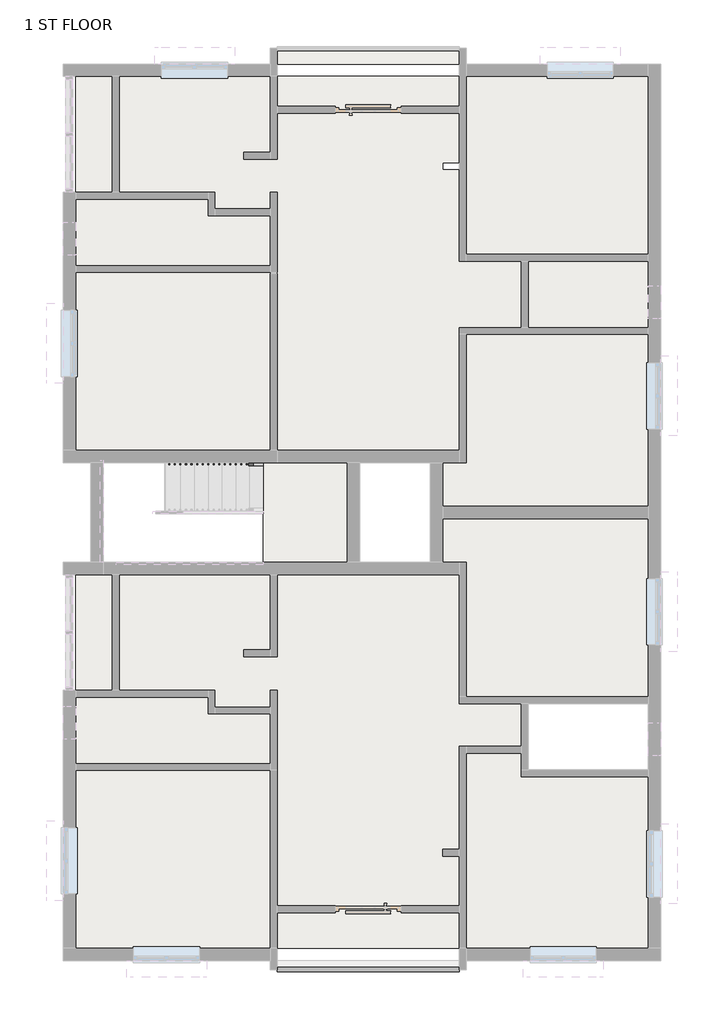
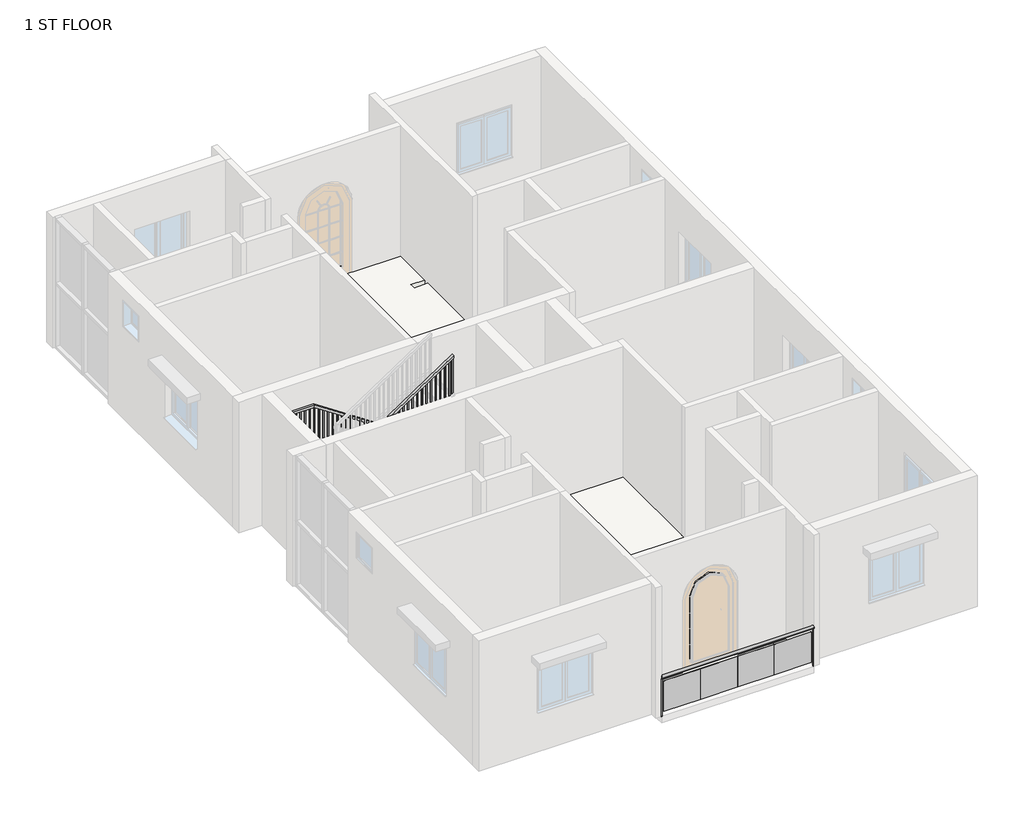
# One storey, part 3 of 4: 4 slabs, 2 railings.
"""IFC4 building model written with IfcOpenShell, lengths in millimetres."""

from ifc_helpers import new_model, si_unit, point, frame, origin, place, context, project, spatial, polyline, ellipse_curve, trimmed, outline, extrude, faceted_brep, element, save
from ifc_brep_helpers import plane_surface, extruded_surface, advanced_brep

model = new_model("IFC4")

# Units and contexts
model_context = context("Model", 3, world=origin())
ifc_project = project(units=[si_unit("LENGTHUNIT", "METRE", prefix="MILLI")], contexts=[model_context])

# Site, building, storey
site = spatial("IfcSite", under=ifc_project)
building = spatial("IfcBuilding", under=site)
storey = spatial("IfcBuildingStorey", under=building, Name="1 ST FLOOR", Elevation=6096.0)

# Railings
placement = place(None, origin())
element("IfcRailing", 1, ObjectType="Glass Panel - Bottom Fill 2", at=placement, inside=storey, context=model_context, shape_type="SolidModel", body=[
    advanced_brep(
    [(-2494.0012202, -3358.1292559, 7010.4), (-2494.0012202, -3434.3292559, 7010.4), (858.7987798, -3358.1292559, 7010.4), (858.7987798, -3434.3292559, 7010.4)],
    [
        (0, 1, ellipse_curve(frame((-2494.0012202, -3396.2292559, 7010.4), z_axis=(-1.0, 0.0, 0.0), x_axis=(0.0, -1.0, 0.0)), 38.1, 28.575)),
        (1, 0, ellipse_curve(frame((-2494.0012202, -3396.2292559, 7010.4), z_axis=(-1.0, 0.0, 0.0), x_axis=(0.0, -1.0, 0.0)), 38.1, 28.575)),
        (2, 3, ellipse_curve(frame((858.7987798, -3396.2292559, 7010.4), z_axis=(1.0, 0.0, 0.0), x_axis=(0.0, -1.0, 0.0)), 38.1, 28.575)),
        (3, 2, ellipse_curve(frame((858.7987798, -3396.2292559, 7010.4), z_axis=(1.0, 0.0, 0.0), x_axis=(0.0, -1.0, 0.0)), 38.1, 28.575)),
        (0, 2),
        (3, 1),
    ],
    [
        plane_surface(frame((-2494.0012202, -3396.2292559, 7010.4), z_axis=(-1.0, 0.0, 0.0), x_axis=(0.0, 1.0, 0.0))),
        plane_surface(frame((858.7987798, -3396.2292559, 7010.4), z_axis=(1.0, 0.0, 0.0), x_axis=(0.0, 1.0, 0.0))),
        extruded_surface(trimmed(ellipse_curve(frame((858.7987798, -3396.2292559, 7010.4), z_axis=(-1.0, 0.0, 0.0), x_axis=(0.0, -1.0, 0.0)), 38.1, 28.575), [point((858.7987798, -3358.1292559, 7010.4))], [point((858.7987798, -3434.3292559, 7010.4))], True, "CARTESIAN"), (-3352.7999999999997, 0.0, 0.0), 3352.7999999999997),
        extruded_surface(trimmed(ellipse_curve(frame((858.7987798, -3396.2292559, 7010.4), z_axis=(-1.0, 0.0, 0.0), x_axis=(0.0, -1.0, 0.0)), 38.1, 28.575), [point((858.7987798, -3434.3292559, 7010.4))], [point((858.7987798, -3358.1292559, 7010.4))], True, "CARTESIAN"), (-3352.7999999999997, 0.0, 0.0), 3352.7999999999997),
    ],
    [
        (0, [[1, 2]]),
        (1, [[3, 4]]),
        (2, [[-1, 5, -4, 6]]),
        (3, [[-2, -6, -3, -5]]),
    ],
),
    extrude(outline(polyline([(-4.8012202, -3402.7644129), (-4.8012202, -3396.4144129), (807.9987798, -3396.4144129), (807.9987798, -3402.7644129), (-4.8012202, -3402.7644129)])), frame((0.0, 0.0, 6197.6), z_axis=(0.0, 0.0, 1.0), x_axis=(1.0, 0.0, 0.0)), (0.0, 0.0, 1.0), 711.2),
    extrude(outline(polyline([(-817.6012202, -3402.7644129), (-817.6012202, -3396.4144129), (-4.8012202, -3396.4144129), (-4.8012202, -3402.7644129), (-817.6012202, -3402.7644129)])), frame((0.0, 0.0, 6197.6), z_axis=(0.0, 0.0, 1.0), x_axis=(1.0, 0.0, 0.0)), (0.0, 0.0, 1.0), 711.2),
    extrude(outline(polyline([(-1630.4012202, -3402.7644129), (-1630.4012202, -3396.4144129), (-817.6012202, -3396.4144129), (-817.6012202, -3402.7644129), (-1630.4012202, -3402.7644129)])), frame((0.0, 0.0, 6197.6), z_axis=(0.0, 0.0, 1.0), x_axis=(1.0, 0.0, 0.0)), (0.0, 0.0, 1.0), 711.2),
    extrude(outline(polyline([(-2443.2012202, -3402.7644129), (-2443.2012202, -3396.4144129), (-1630.4012202, -3396.4144129), (-1630.4012202, -3402.7644129), (-2443.2012202, -3402.7644129)])), frame((0.0, 0.0, 6197.6), z_axis=(0.0, 0.0, 1.0), x_axis=(1.0, 0.0, 0.0)), (0.0, 0.0, 1.0), 711.2),
    extrude(outline(polyline([(846.0987798, -3386.7042559), (865.1487798, -3386.7042559), (865.1487798, -3405.7542559), (846.0987798, -3405.7542559), (846.0987798, -3386.7042559)])), frame((0.0, 0.0, 6096.0), z_axis=(0.0, 0.0, 1.0), x_axis=(1.0, 0.0, 0.0)), (0.0, 0.0, 1.0), 885.825),
    extrude(outline(polyline([(-2500.3512202, -3386.7042559), (-2481.3012202, -3386.7042559), (-2481.3012202, -3405.7542559), (-2500.3512202, -3405.7542559), (-2500.3512202, -3386.7042559)])), frame((0.0, 0.0, 6096.0), z_axis=(0.0, 0.0, 1.0), x_axis=(1.0, 0.0, 0.0)), (0.0, 0.0, 1.0), 885.825),
])
element("IfcRailing", 2, ObjectType="Handrail - Rectangular", at=placement, inside=storey, context=model_context, shape_type="SolidModel", body=[
    faceted_brep([(-2748.0012202, 5879.8309003, 7179.7333333), (-2748.0012202, 5879.8309003, 7118.6793317), (-2748.0012202, 5930.6309003, 7118.6793317), (-2748.0012202, 5930.6309003, 7179.7333333), (-4780.0012202, 5879.8309003, 8534.4), (-4795.3822226, 5879.8309003, 8483.6), (-4795.3822226, 5930.6309003, 8483.6), (-4780.0012202, 5930.6309003, 8534.4), (-5643.6012202, 5879.8309003, 8534.4), (-5643.6012202, 5879.8309003, 8483.6), (-5694.4012202, 5930.6309003, 8483.6), (-5694.4012202, 5930.6309003, 8534.4), (-5643.6012202, 4152.6309003, 8534.4), (-5643.6012202, 4152.6309003, 8483.6), (-5694.4012202, 4101.8309003, 8483.6), (-5694.4012202, 4101.8309003, 8534.4), (-5034.0012202, 4152.6309003, 8534.4), (-5018.6202178, 4152.6309003, 8483.6), (-5018.6202178, 4101.8309003, 8483.6), (-5034.0012202, 4101.8309003, 8534.4), (-2748.0012202, 4152.6309003, 10058.4), (-2748.0012202, 4101.8309003, 10058.4), (-2748.0012202, 4101.8309003, 9997.3459984), (-2748.0012202, 4152.6309003, 9997.3459984)], [[[0, 1, 2, 3]], [[1, 0, 4, 5]], [[2, 1, 5, 6]], [[3, 2, 6, 7]], [[0, 3, 7, 4]], [[5, 4, 8, 9]], [[6, 5, 9, 10]], [[7, 6, 10, 11]], [[4, 7, 11, 8]], [[9, 8, 12, 13]], [[10, 9, 13, 14]], [[11, 10, 14, 15]], [[8, 11, 15, 12]], [[13, 12, 16, 17]], [[14, 13, 17, 18]], [[15, 14, 18, 19]], [[12, 15, 19, 16]], [[20, 21, 22, 23]], [[17, 16, 20, 23]], [[18, 17, 23, 22]], [[19, 18, 22, 21]], [[16, 19, 21, 20]]]),
    extrude(outline(polyline([(9952.8959984, -2814.6762202), (9940.1959984, -2833.7262202), (8974.6666667, -2833.7262202), (8974.6666667, -2814.6762202), (9952.8959984, -2814.6762202)])), frame((0.0, 4117.7059003, 0.0), z_axis=(0.0, 1.0, 0.0), x_axis=(0.0, 0.0, 1.0)), (0.0, 0.0, 1.0), 19.05),
    extrude(outline(polyline([(9885.1626651, -2916.2762202), (9872.4626651, -2935.3262202), (8974.6666667, -2935.3262202), (8974.6666667, -2916.2762202), (9885.1626651, -2916.2762202)])), frame((0.0, 4117.7059003, 0.0), z_axis=(0.0, 1.0, 0.0), x_axis=(0.0, 0.0, 1.0)), (0.0, 0.0, 1.0), 19.05),
    extrude(outline(polyline([(9817.4293317, -3017.8762202), (9804.7293317, -3036.9262202), (8805.3333333, -3036.9262202), (8805.3333333, -3017.8762202), (9817.4293317, -3017.8762202)])), frame((0.0, 4117.7059003, 0.0), z_axis=(0.0, 1.0, 0.0), x_axis=(0.0, 0.0, 1.0)), (0.0, 0.0, 1.0), 19.05),
    extrude(outline(polyline([(9749.6959984, -3119.4762202), (9736.9959984, -3138.5262202), (8805.3333333, -3138.5262202), (8805.3333333, -3119.4762202), (9749.6959984, -3119.4762202)])), frame((0.0, 4117.7059003, 0.0), z_axis=(0.0, 1.0, 0.0), x_axis=(0.0, 0.0, 1.0)), (0.0, 0.0, 1.0), 19.05),
    extrude(outline(polyline([(9681.9626651, -3221.0762202), (9669.2626651, -3240.1262202), (8805.3333333, -3240.1262202), (8805.3333333, -3221.0762202), (9681.9626651, -3221.0762202)])), frame((0.0, 4117.7059003, 0.0), z_axis=(0.0, 1.0, 0.0), x_axis=(0.0, 0.0, 1.0)), (0.0, 0.0, 1.0), 19.05),
    extrude(outline(polyline([(9614.2293317, -3322.6762202), (9601.5293317, -3341.7262202), (8636.0, -3341.7262202), (8636.0, -3322.6762202), (9614.2293317, -3322.6762202)])), frame((0.0, 4117.7059003, 0.0), z_axis=(0.0, 1.0, 0.0), x_axis=(0.0, 0.0, 1.0)), (0.0, 0.0, 1.0), 19.05),
    extrude(outline(polyline([(9546.4959984, -3424.2762202), (9533.7959984, -3443.3262202), (8636.0, -3443.3262202), (8636.0, -3424.2762202), (9546.4959984, -3424.2762202)])), frame((0.0, 4117.7059003, 0.0), z_axis=(0.0, 1.0, 0.0), x_axis=(0.0, 0.0, 1.0)), (0.0, 0.0, 1.0), 19.05),
    extrude(outline(polyline([(9478.7626651, -3525.8762202), (9466.0626651, -3544.9262202), (8466.6666667, -3544.9262202), (8466.6666667, -3525.8762202), (9478.7626651, -3525.8762202)])), frame((0.0, 4117.7059003, 0.0), z_axis=(0.0, 1.0, 0.0), x_axis=(0.0, 0.0, 1.0)), (0.0, 0.0, 1.0), 19.05),
    extrude(outline(polyline([(9411.0293317, -3627.4762202), (9398.3293317, -3646.5262202), (8466.6666667, -3646.5262202), (8466.6666667, -3627.4762202), (9411.0293317, -3627.4762202)])), frame((0.0, 4117.7059003, 0.0), z_axis=(0.0, 1.0, 0.0), x_axis=(0.0, 0.0, 1.0)), (0.0, 0.0, 1.0), 19.05),
    extrude(outline(polyline([(9343.2959984, -3729.0762202), (9330.5959984, -3748.1262202), (8466.6666667, -3748.1262202), (8466.6666667, -3729.0762202), (9343.2959984, -3729.0762202)])), frame((0.0, 4117.7059003, 0.0), z_axis=(0.0, 1.0, 0.0), x_axis=(0.0, 0.0, 1.0)), (0.0, 0.0, 1.0), 19.05),
    extrude(outline(polyline([(9275.5626651, -3830.6762202), (9262.8626651, -3849.7262202), (8297.3333333, -3849.7262202), (8297.3333333, -3830.6762202), (9275.5626651, -3830.6762202)])), frame((0.0, 4117.7059003, 0.0), z_axis=(0.0, 1.0, 0.0), x_axis=(0.0, 0.0, 1.0)), (0.0, 0.0, 1.0), 19.05),
    extrude(outline(polyline([(9207.8293317, -3932.2762202), (9195.1293317, -3951.3262202), (8297.3333333, -3951.3262202), (8297.3333333, -3932.2762202), (9207.8293317, -3932.2762202)])), frame((0.0, 4117.7059003, 0.0), z_axis=(0.0, 1.0, 0.0), x_axis=(0.0, 0.0, 1.0)), (0.0, 0.0, 1.0), 19.05),
    extrude(outline(polyline([(9140.0959984, -4033.8762202), (9127.3959984, -4052.9262202), (8128.0, -4052.9262202), (8128.0, -4033.8762202), (9140.0959984, -4033.8762202)])), frame((0.0, 4117.7059003, 0.0), z_axis=(0.0, 1.0, 0.0), x_axis=(0.0, 0.0, 1.0)), (0.0, 0.0, 1.0), 19.05),
    extrude(outline(polyline([(9072.3626651, -4135.4762202), (9059.6626651, -4154.5262202), (8128.0, -4154.5262202), (8128.0, -4135.4762202), (9072.3626651, -4135.4762202)])), frame((0.0, 4117.7059003, 0.0), z_axis=(0.0, 1.0, 0.0), x_axis=(0.0, 0.0, 1.0)), (0.0, 0.0, 1.0), 19.05),
    extrude(outline(polyline([(9004.6293317, -4237.0762202), (8991.9293317, -4256.1262202), (8128.0, -4256.1262202), (8128.0, -4237.0762202), (9004.6293317, -4237.0762202)])), frame((0.0, 4117.7059003, 0.0), z_axis=(0.0, 1.0, 0.0), x_axis=(0.0, 0.0, 1.0)), (0.0, 0.0, 1.0), 19.05),
    extrude(outline(polyline([(8936.8959984, -4338.6762202), (8924.1959984, -4357.7262202), (7958.6666667, -4357.7262202), (7958.6666667, -4338.6762202), (8936.8959984, -4338.6762202)])), frame((0.0, 4117.7059003, 0.0), z_axis=(0.0, 1.0, 0.0), x_axis=(0.0, 0.0, 1.0)), (0.0, 0.0, 1.0), 19.05),
    extrude(outline(polyline([(8869.1626651, -4440.2762202), (8856.4626651, -4459.3262202), (7958.6666667, -4459.3262202), (7958.6666667, -4440.2762202), (8869.1626651, -4440.2762202)])), frame((0.0, 4117.7059003, 0.0), z_axis=(0.0, 1.0, 0.0), x_axis=(0.0, 0.0, 1.0)), (0.0, 0.0, 1.0), 19.05),
    extrude(outline(polyline([(8801.4293317, -4541.8762202), (8788.7293317, -4560.9262202), (7789.3333333, -4560.9262202), (7789.3333333, -4541.8762202), (8801.4293317, -4541.8762202)])), frame((0.0, 4117.7059003, 0.0), z_axis=(0.0, 1.0, 0.0), x_axis=(0.0, 0.0, 1.0)), (0.0, 0.0, 1.0), 19.05),
    extrude(outline(polyline([(8733.6959984, -4643.4762202), (8720.9959984, -4662.5262202), (7789.3333333, -4662.5262202), (7789.3333333, -4643.4762202), (8733.6959984, -4643.4762202)])), frame((0.0, 4117.7059003, 0.0), z_axis=(0.0, 1.0, 0.0), x_axis=(0.0, 0.0, 1.0)), (0.0, 0.0, 1.0), 19.05),
    extrude(outline(polyline([(8665.9626651, -4745.0762202), (8653.2626651, -4764.1262202), (7789.3333333, -4764.1262202), (7789.3333333, -4745.0762202), (8665.9626651, -4745.0762202)])), frame((0.0, 4117.7059003, 0.0), z_axis=(0.0, 1.0, 0.0), x_axis=(0.0, 0.0, 1.0)), (0.0, 0.0, 1.0), 19.05),
    extrude(outline(polyline([(8598.2293317, -4846.6762202), (8585.5293317, -4865.7262202), (7620.0, -4865.7262202), (7620.0, -4846.6762202), (8598.2293317, -4846.6762202)])), frame((0.0, 4117.7059003, 0.0), z_axis=(0.0, 1.0, 0.0), x_axis=(0.0, 0.0, 1.0)), (0.0, 0.0, 1.0), 19.05),
    extrude(outline(polyline([(8530.4959984, -4948.2762202), (8517.7959984, -4967.3262202), (7620.0, -4967.3262202), (7620.0, -4948.2762202), (8530.4959984, -4948.2762202)])), frame((0.0, 4117.7059003, 0.0), z_axis=(0.0, 1.0, 0.0), x_axis=(0.0, 0.0, 1.0)), (0.0, 0.0, 1.0), 19.05),
    extrude(outline(polyline([(-5068.9262202, 4117.7059003), (-5068.9262202, 4136.7559003), (-5049.8762202, 4136.7559003), (-5049.8762202, 4117.7059003), (-5068.9262202, 4117.7059003)])), frame((0.0, 0.0, 7620.0), z_axis=(0.0, 0.0, 1.0), x_axis=(1.0, 0.0, 0.0)), (0.0, 0.0, 1.0), 863.6),
    extrude(outline(polyline([(-5170.5262202, 4117.7059003), (-5170.5262202, 4136.7559003), (-5151.4762202, 4136.7559003), (-5151.4762202, 4117.7059003), (-5170.5262202, 4117.7059003)])), frame((0.0, 0.0, 7620.0), z_axis=(0.0, 0.0, 1.0), x_axis=(1.0, 0.0, 0.0)), (0.0, 0.0, 1.0), 863.6),
    extrude(outline(polyline([(-5272.1262202, 4117.7059003), (-5272.1262202, 4136.7559003), (-5253.0762202, 4136.7559003), (-5253.0762202, 4117.7059003), (-5272.1262202, 4117.7059003)])), frame((0.0, 0.0, 7620.0), z_axis=(0.0, 0.0, 1.0), x_axis=(1.0, 0.0, 0.0)), (0.0, 0.0, 1.0), 863.6),
    extrude(outline(polyline([(-5373.7262202, 4117.7059003), (-5373.7262202, 4136.7559003), (-5354.6762202, 4136.7559003), (-5354.6762202, 4117.7059003), (-5373.7262202, 4117.7059003)])), frame((0.0, 0.0, 7620.0), z_axis=(0.0, 0.0, 1.0), x_axis=(1.0, 0.0, 0.0)), (0.0, 0.0, 1.0), 863.6),
    extrude(outline(polyline([(-5475.3262202, 4117.7059003), (-5475.3262202, 4136.7559003), (-5456.2762202, 4136.7559003), (-5456.2762202, 4117.7059003), (-5475.3262202, 4117.7059003)])), frame((0.0, 0.0, 7620.0), z_axis=(0.0, 0.0, 1.0), x_axis=(1.0, 0.0, 0.0)), (0.0, 0.0, 1.0), 863.6),
    extrude(outline(polyline([(-5576.9262202, 4117.7059003), (-5576.9262202, 4136.7559003), (-5557.8762202, 4136.7559003), (-5557.8762202, 4117.7059003), (-5576.9262202, 4117.7059003)])), frame((0.0, 0.0, 7620.0), z_axis=(0.0, 0.0, 1.0), x_axis=(1.0, 0.0, 0.0)), (0.0, 0.0, 1.0), 863.6),
    extrude(outline(polyline([(-5678.5262202, 4187.5559003), (-5659.4762202, 4187.5559003), (-5659.4762202, 4168.5059003), (-5678.5262202, 4168.5059003), (-5678.5262202, 4187.5559003)])), frame((0.0, 0.0, 7620.0), z_axis=(0.0, 0.0, 1.0), x_axis=(1.0, 0.0, 0.0)), (0.0, 0.0, 1.0), 863.6),
    extrude(outline(polyline([(-5678.5262202, 4289.1559003), (-5659.4762202, 4289.1559003), (-5659.4762202, 4270.1059003), (-5678.5262202, 4270.1059003), (-5678.5262202, 4289.1559003)])), frame((0.0, 0.0, 7620.0), z_axis=(0.0, 0.0, 1.0), x_axis=(1.0, 0.0, 0.0)), (0.0, 0.0, 1.0), 863.6),
    extrude(outline(polyline([(-5678.5262202, 4390.7559003), (-5659.4762202, 4390.7559003), (-5659.4762202, 4371.7059003), (-5678.5262202, 4371.7059003), (-5678.5262202, 4390.7559003)])), frame((0.0, 0.0, 7620.0), z_axis=(0.0, 0.0, 1.0), x_axis=(1.0, 0.0, 0.0)), (0.0, 0.0, 1.0), 863.6),
    extrude(outline(polyline([(-5678.5262202, 4492.3559003), (-5659.4762202, 4492.3559003), (-5659.4762202, 4473.3059003), (-5678.5262202, 4473.3059003), (-5678.5262202, 4492.3559003)])), frame((0.0, 0.0, 7620.0), z_axis=(0.0, 0.0, 1.0), x_axis=(1.0, 0.0, 0.0)), (0.0, 0.0, 1.0), 863.6),
    extrude(outline(polyline([(-5678.5262202, 4593.9559003), (-5659.4762202, 4593.9559003), (-5659.4762202, 4574.9059003), (-5678.5262202, 4574.9059003), (-5678.5262202, 4593.9559003)])), frame((0.0, 0.0, 7620.0), z_axis=(0.0, 0.0, 1.0), x_axis=(1.0, 0.0, 0.0)), (0.0, 0.0, 1.0), 863.6),
    extrude(outline(polyline([(-5678.5262202, 4695.5559003), (-5659.4762202, 4695.5559003), (-5659.4762202, 4676.5059003), (-5678.5262202, 4676.5059003), (-5678.5262202, 4695.5559003)])), frame((0.0, 0.0, 7620.0), z_axis=(0.0, 0.0, 1.0), x_axis=(1.0, 0.0, 0.0)), (0.0, 0.0, 1.0), 863.6),
    extrude(outline(polyline([(-5678.5262202, 4797.1559003), (-5659.4762202, 4797.1559003), (-5659.4762202, 4778.1059003), (-5678.5262202, 4778.1059003), (-5678.5262202, 4797.1559003)])), frame((0.0, 0.0, 7620.0), z_axis=(0.0, 0.0, 1.0), x_axis=(1.0, 0.0, 0.0)), (0.0, 0.0, 1.0), 863.6),
    extrude(outline(polyline([(-5678.5262202, 4898.7559003), (-5659.4762202, 4898.7559003), (-5659.4762202, 4879.7059003), (-5678.5262202, 4879.7059003), (-5678.5262202, 4898.7559003)])), frame((0.0, 0.0, 7620.0), z_axis=(0.0, 0.0, 1.0), x_axis=(1.0, 0.0, 0.0)), (0.0, 0.0, 1.0), 863.6),
    extrude(outline(polyline([(-5678.5262202, 5000.3559003), (-5659.4762202, 5000.3559003), (-5659.4762202, 4981.3059003), (-5678.5262202, 4981.3059003), (-5678.5262202, 5000.3559003)])), frame((0.0, 0.0, 7620.0), z_axis=(0.0, 0.0, 1.0), x_axis=(1.0, 0.0, 0.0)), (0.0, 0.0, 1.0), 863.6),
    extrude(outline(polyline([(-5678.5262202, 5101.9559003), (-5659.4762202, 5101.9559003), (-5659.4762202, 5082.9059003), (-5678.5262202, 5082.9059003), (-5678.5262202, 5101.9559003)])), frame((0.0, 0.0, 7620.0), z_axis=(0.0, 0.0, 1.0), x_axis=(1.0, 0.0, 0.0)), (0.0, 0.0, 1.0), 863.6),
    extrude(outline(polyline([(-5678.5262202, 5203.5559003), (-5659.4762202, 5203.5559003), (-5659.4762202, 5184.5059003), (-5678.5262202, 5184.5059003), (-5678.5262202, 5203.5559003)])), frame((0.0, 0.0, 7620.0), z_axis=(0.0, 0.0, 1.0), x_axis=(1.0, 0.0, 0.0)), (0.0, 0.0, 1.0), 863.6),
    extrude(outline(polyline([(-5678.5262202, 5305.1559003), (-5659.4762202, 5305.1559003), (-5659.4762202, 5286.1059003), (-5678.5262202, 5286.1059003), (-5678.5262202, 5305.1559003)])), frame((0.0, 0.0, 7620.0), z_axis=(0.0, 0.0, 1.0), x_axis=(1.0, 0.0, 0.0)), (0.0, 0.0, 1.0), 863.6),
    extrude(outline(polyline([(-5678.5262202, 5406.7559003), (-5659.4762202, 5406.7559003), (-5659.4762202, 5387.7059003), (-5678.5262202, 5387.7059003), (-5678.5262202, 5406.7559003)])), frame((0.0, 0.0, 7620.0), z_axis=(0.0, 0.0, 1.0), x_axis=(1.0, 0.0, 0.0)), (0.0, 0.0, 1.0), 863.6),
    extrude(outline(polyline([(-5678.5262202, 5508.3559003), (-5659.4762202, 5508.3559003), (-5659.4762202, 5489.3059003), (-5678.5262202, 5489.3059003), (-5678.5262202, 5508.3559003)])), frame((0.0, 0.0, 7620.0), z_axis=(0.0, 0.0, 1.0), x_axis=(1.0, 0.0, 0.0)), (0.0, 0.0, 1.0), 863.6),
    extrude(outline(polyline([(-5678.5262202, 5609.9559003), (-5659.4762202, 5609.9559003), (-5659.4762202, 5590.9059003), (-5678.5262202, 5590.9059003), (-5678.5262202, 5609.9559003)])), frame((0.0, 0.0, 7620.0), z_axis=(0.0, 0.0, 1.0), x_axis=(1.0, 0.0, 0.0)), (0.0, 0.0, 1.0), 863.6),
    extrude(outline(polyline([(-5678.5262202, 5711.5559003), (-5659.4762202, 5711.5559003), (-5659.4762202, 5692.5059003), (-5678.5262202, 5692.5059003), (-5678.5262202, 5711.5559003)])), frame((0.0, 0.0, 7620.0), z_axis=(0.0, 0.0, 1.0), x_axis=(1.0, 0.0, 0.0)), (0.0, 0.0, 1.0), 863.6),
    extrude(outline(polyline([(-5678.5262202, 5813.1559003), (-5659.4762202, 5813.1559003), (-5659.4762202, 5794.1059003), (-5678.5262202, 5794.1059003), (-5678.5262202, 5813.1559003)])), frame((0.0, 0.0, 7620.0), z_axis=(0.0, 0.0, 1.0), x_axis=(1.0, 0.0, 0.0)), (0.0, 0.0, 1.0), 863.6),
    extrude(outline(polyline([(-5583.2762202, 5914.7559003), (-5583.2762202, 5895.7059003), (-5602.3262202, 5895.7059003), (-5602.3262202, 5914.7559003), (-5583.2762202, 5914.7559003)])), frame((0.0, 0.0, 7620.0), z_axis=(0.0, 0.0, 1.0), x_axis=(1.0, 0.0, 0.0)), (0.0, 0.0, 1.0), 863.6),
    extrude(outline(polyline([(-5481.6762202, 5914.7559003), (-5481.6762202, 5895.7059003), (-5500.7262202, 5895.7059003), (-5500.7262202, 5914.7559003), (-5481.6762202, 5914.7559003)])), frame((0.0, 0.0, 7620.0), z_axis=(0.0, 0.0, 1.0), x_axis=(1.0, 0.0, 0.0)), (0.0, 0.0, 1.0), 863.6),
    extrude(outline(polyline([(-5380.0762202, 5914.7559003), (-5380.0762202, 5895.7059003), (-5399.1262202, 5895.7059003), (-5399.1262202, 5914.7559003), (-5380.0762202, 5914.7559003)])), frame((0.0, 0.0, 7620.0), z_axis=(0.0, 0.0, 1.0), x_axis=(1.0, 0.0, 0.0)), (0.0, 0.0, 1.0), 863.6),
    extrude(outline(polyline([(-5278.4762202, 5914.7559003), (-5278.4762202, 5895.7059003), (-5297.5262202, 5895.7059003), (-5297.5262202, 5914.7559003), (-5278.4762202, 5914.7559003)])), frame((0.0, 0.0, 7620.0), z_axis=(0.0, 0.0, 1.0), x_axis=(1.0, 0.0, 0.0)), (0.0, 0.0, 1.0), 863.6),
    extrude(outline(polyline([(-5176.8762202, 5914.7559003), (-5176.8762202, 5895.7059003), (-5195.9262202, 5895.7059003), (-5195.9262202, 5914.7559003), (-5176.8762202, 5914.7559003)])), frame((0.0, 0.0, 7620.0), z_axis=(0.0, 0.0, 1.0), x_axis=(1.0, 0.0, 0.0)), (0.0, 0.0, 1.0), 863.6),
    extrude(outline(polyline([(-5075.2762202, 5914.7559003), (-5075.2762202, 5895.7059003), (-5094.3262202, 5895.7059003), (-5094.3262202, 5914.7559003), (-5075.2762202, 5914.7559003)])), frame((0.0, 0.0, 7620.0), z_axis=(0.0, 0.0, 1.0), x_axis=(1.0, 0.0, 0.0)), (0.0, 0.0, 1.0), 863.6),
    extrude(outline(polyline([(-4973.6762202, 5914.7559003), (-4973.6762202, 5895.7059003), (-4992.7262202, 5895.7059003), (-4992.7262202, 5914.7559003), (-4973.6762202, 5914.7559003)])), frame((0.0, 0.0, 7620.0), z_axis=(0.0, 0.0, 1.0), x_axis=(1.0, 0.0, 0.0)), (0.0, 0.0, 1.0), 863.6),
    extrude(outline(polyline([(-4872.0762202, 5914.7559003), (-4872.0762202, 5895.7059003), (-4891.1262202, 5895.7059003), (-4891.1262202, 5914.7559003), (-4872.0762202, 5914.7559003)])), frame((0.0, 0.0, 7620.0), z_axis=(0.0, 0.0, 1.0), x_axis=(1.0, 0.0, 0.0)), (0.0, 0.0, 1.0), 863.6),
    extrude(outline(polyline([(8466.9959984, -4770.4762202), (8479.6959984, -4789.5262202), (7620.0, -4789.5262202), (7620.0, -4770.4762202), (8466.9959984, -4770.4762202)])), frame((0.0, 5895.7059003, 0.0), z_axis=(0.0, 1.0, 0.0), x_axis=(0.0, 0.0, 1.0)), (0.0, 0.0, 1.0), 19.05),
    extrude(outline(polyline([(8399.2626651, -4668.8762202), (8411.9626651, -4687.9262202), (7450.6666667, -4687.9262202), (7450.6666667, -4668.8762202), (8399.2626651, -4668.8762202)])), frame((0.0, 5895.7059003, 0.0), z_axis=(0.0, 1.0, 0.0), x_axis=(0.0, 0.0, 1.0)), (0.0, 0.0, 1.0), 19.05),
    extrude(outline(polyline([(8331.5293317, -4567.2762202), (8344.2293317, -4586.3262202), (7450.6666667, -4586.3262202), (7450.6666667, -4567.2762202), (8331.5293317, -4567.2762202)])), frame((0.0, 5895.7059003, 0.0), z_axis=(0.0, 1.0, 0.0), x_axis=(0.0, 0.0, 1.0)), (0.0, 0.0, 1.0), 19.05),
    extrude(outline(polyline([(8263.7959984, -4465.6762202), (8276.4959984, -4484.7262202), (7281.3333333, -4484.7262202), (7281.3333333, -4465.6762202), (8263.7959984, -4465.6762202)])), frame((0.0, 5895.7059003, 0.0), z_axis=(0.0, 1.0, 0.0), x_axis=(0.0, 0.0, 1.0)), (0.0, 0.0, 1.0), 19.05),
    extrude(outline(polyline([(8196.0626651, -4364.0762202), (8208.7626651, -4383.1262202), (7281.3333333, -4383.1262202), (7281.3333333, -4364.0762202), (8196.0626651, -4364.0762202)])), frame((0.0, 5895.7059003, 0.0), z_axis=(0.0, 1.0, 0.0), x_axis=(0.0, 0.0, 1.0)), (0.0, 0.0, 1.0), 19.05),
    extrude(outline(polyline([(8128.3293317, -4262.4762202), (8141.0293317, -4281.5262202), (7281.3333333, -4281.5262202), (7281.3333333, -4262.4762202), (8128.3293317, -4262.4762202)])), frame((0.0, 5895.7059003, 0.0), z_axis=(0.0, 1.0, 0.0), x_axis=(0.0, 0.0, 1.0)), (0.0, 0.0, 1.0), 19.05),
    extrude(outline(polyline([(8060.5959984, -4160.8762202), (8073.2959984, -4179.9262202), (7112.0, -4179.9262202), (7112.0, -4160.8762202), (8060.5959984, -4160.8762202)])), frame((0.0, 5895.7059003, 0.0), z_axis=(0.0, 1.0, 0.0), x_axis=(0.0, 0.0, 1.0)), (0.0, 0.0, 1.0), 19.05),
    extrude(outline(polyline([(7992.8626651, -4059.2762202), (8005.5626651, -4078.3262202), (7112.0, -4078.3262202), (7112.0, -4059.2762202), (7992.8626651, -4059.2762202)])), frame((0.0, 5895.7059003, 0.0), z_axis=(0.0, 1.0, 0.0), x_axis=(0.0, 0.0, 1.0)), (0.0, 0.0, 1.0), 19.05),
    extrude(outline(polyline([(7925.1293317, -3957.6762202), (7937.8293317, -3976.7262202), (6942.6666667, -3976.7262202), (6942.6666667, -3957.6762202), (7925.1293317, -3957.6762202)])), frame((0.0, 5895.7059003, 0.0), z_axis=(0.0, 1.0, 0.0), x_axis=(0.0, 0.0, 1.0)), (0.0, 0.0, 1.0), 19.05),
    extrude(outline(polyline([(7857.3959984, -3856.0762202), (7870.0959984, -3875.1262202), (6942.6666667, -3875.1262202), (6942.6666667, -3856.0762202), (7857.3959984, -3856.0762202)])), frame((0.0, 5895.7059003, 0.0), z_axis=(0.0, 1.0, 0.0), x_axis=(0.0, 0.0, 1.0)), (0.0, 0.0, 1.0), 19.05),
    extrude(outline(polyline([(7789.6626651, -3754.4762202), (7802.3626651, -3773.5262202), (6942.6666667, -3773.5262202), (6942.6666667, -3754.4762202), (7789.6626651, -3754.4762202)])), frame((0.0, 5895.7059003, 0.0), z_axis=(0.0, 1.0, 0.0), x_axis=(0.0, 0.0, 1.0)), (0.0, 0.0, 1.0), 19.05),
    extrude(outline(polyline([(7721.9293317, -3652.8762202), (7734.6293317, -3671.9262202), (6773.3333333, -3671.9262202), (6773.3333333, -3652.8762202), (7721.9293317, -3652.8762202)])), frame((0.0, 5895.7059003, 0.0), z_axis=(0.0, 1.0, 0.0), x_axis=(0.0, 0.0, 1.0)), (0.0, 0.0, 1.0), 19.05),
    extrude(outline(polyline([(7654.1959984, -3551.2762202), (7666.8959984, -3570.3262202), (6773.3333333, -3570.3262202), (6773.3333333, -3551.2762202), (7654.1959984, -3551.2762202)])), frame((0.0, 5895.7059003, 0.0), z_axis=(0.0, 1.0, 0.0), x_axis=(0.0, 0.0, 1.0)), (0.0, 0.0, 1.0), 19.05),
    extrude(outline(polyline([(7586.4626651, -3449.6762202), (7599.1626651, -3468.7262202), (6604.0, -3468.7262202), (6604.0, -3449.6762202), (7586.4626651, -3449.6762202)])), frame((0.0, 5895.7059003, 0.0), z_axis=(0.0, 1.0, 0.0), x_axis=(0.0, 0.0, 1.0)), (0.0, 0.0, 1.0), 19.05),
    extrude(outline(polyline([(7518.7293317, -3348.0762202), (7531.4293317, -3367.1262202), (6604.0, -3367.1262202), (6604.0, -3348.0762202), (7518.7293317, -3348.0762202)])), frame((0.0, 5895.7059003, 0.0), z_axis=(0.0, 1.0, 0.0), x_axis=(0.0, 0.0, 1.0)), (0.0, 0.0, 1.0), 19.05),
    extrude(outline(polyline([(7450.9959984, -3246.4762202), (7463.6959984, -3265.5262202), (6604.0, -3265.5262202), (6604.0, -3246.4762202), (7450.9959984, -3246.4762202)])), frame((0.0, 5895.7059003, 0.0), z_axis=(0.0, 1.0, 0.0), x_axis=(0.0, 0.0, 1.0)), (0.0, 0.0, 1.0), 19.05),
    extrude(outline(polyline([(7383.2626651, -3144.8762202), (7395.9626651, -3163.9262202), (6434.6666667, -3163.9262202), (6434.6666667, -3144.8762202), (7383.2626651, -3144.8762202)])), frame((0.0, 5895.7059003, 0.0), z_axis=(0.0, 1.0, 0.0), x_axis=(0.0, 0.0, 1.0)), (0.0, 0.0, 1.0), 19.05),
    extrude(outline(polyline([(7315.5293317, -3043.2762202), (7328.2293317, -3062.3262202), (6434.6666667, -3062.3262202), (6434.6666667, -3043.2762202), (7315.5293317, -3043.2762202)])), frame((0.0, 5895.7059003, 0.0), z_axis=(0.0, 1.0, 0.0), x_axis=(0.0, 0.0, 1.0)), (0.0, 0.0, 1.0), 19.05),
    extrude(outline(polyline([(7247.7959984, -2941.6762202), (7260.4959984, -2960.7262202), (6265.3333333, -2960.7262202), (6265.3333333, -2941.6762202), (7247.7959984, -2941.6762202)])), frame((0.0, 5895.7059003, 0.0), z_axis=(0.0, 1.0, 0.0), x_axis=(0.0, 0.0, 1.0)), (0.0, 0.0, 1.0), 19.05),
    extrude(outline(polyline([(7180.0626651, -2840.0762202), (7192.7626651, -2859.1262202), (6265.3333333, -2859.1262202), (6265.3333333, -2840.0762202), (7180.0626651, -2840.0762202)])), frame((0.0, 5895.7059003, 0.0), z_axis=(0.0, 1.0, 0.0), x_axis=(0.0, 0.0, 1.0)), (0.0, 0.0, 1.0), 19.05),
    extrude(outline(polyline([(-5678.5262202, 4136.7559003), (-5659.4762202, 4136.7559003), (-5659.4762202, 4117.7059003), (-5678.5262202, 4117.7059003), (-5678.5262202, 4136.7559003)])), frame((0.0, 0.0, 7620.0), z_axis=(0.0, 0.0, 1.0), x_axis=(1.0, 0.0, 0.0)), (0.0, 0.0, 1.0), 863.6),
    extrude(outline(polyline([(-5659.4762202, 5914.7559003), (-5659.4762202, 5895.7059003), (-5678.5262202, 5895.7059003), (-5678.5262202, 5914.7559003), (-5659.4762202, 5914.7559003)])), frame((0.0, 0.0, 7620.0), z_axis=(0.0, 0.0, 1.0), x_axis=(1.0, 0.0, 0.0)), (0.0, 0.0, 1.0), 863.6),
    extrude(outline(polyline([(9997.3459984, -2748.0012202), (9984.6459984, -2767.0512202), (8974.6666667, -2767.0512202), (8974.6666667, -2748.0012202), (9997.3459984, -2748.0012202)])), frame((0.0, 4117.7059003, 0.0), z_axis=(0.0, 1.0, 0.0), x_axis=(0.0, 0.0, 1.0)), (0.0, 0.0, 1.0), 19.05),
    extrude(outline(polyline([(7118.6793317, -2748.0012202), (7131.3793317, -2767.0512202), (6265.3333333, -2767.0512202), (6265.3333333, -2748.0012202), (7118.6793317, -2748.0012202)])), frame((0.0, 5895.7059003, 0.0), z_axis=(0.0, 1.0, 0.0), x_axis=(0.0, 0.0, 1.0)), (0.0, 0.0, 1.0), 19.05),
])

# Slabs
element("IfcSlab", 3, ObjectType="FLOORING 6\"", at=placement, inside=storey, context=model_context, shape_type="SweptSolid", body=[
    extrude(outline(polyline([(-2621.0012202, 11645.6309003), (-3103.6012202, 11645.6309003), (-3103.6012202, 11518.6309003), (-2557.5012202, 11518.6309003), (-2494.0012202, 11518.6309003), (-2494.0012202, 13042.6309003), (858.7987798, 13042.6309003), (858.7987798, 11455.1309003), (553.9987798, 11455.1309003), (553.9987798, 11328.1309003), (858.7987798, 11328.1309003), (858.7987798, 9639.0309003), (2001.7987798, 9639.0309003), (2001.7987798, 8419.8309003), (858.7987798, 8419.8309003), (858.7987798, 6159.2309003), (-2494.0012202, 6159.2309003), (-2494.0012202, 9435.8309003), (-2494.0012202, 10909.0309003), (-2621.0012202, 10909.0309003), (-2621.0012202, 10604.2309003), (-3637.0012202, 10604.2309003), (-3637.0012202, 10909.0309003), (-6202.4012202, 10909.0309003), (-6202.4012202, 13042.6309003), (-2621.0012202, 13042.6309003), (-2621.0012202, 11645.6309003)])), frame((0.0, 0.0, 5943.6), z_axis=(0.0, 0.0, 1.0), x_axis=(1.0, 0.0, 0.0)), (0.0, 0.0, 1.0), 152.4),
])
element("IfcSlab", 4, ObjectType="FLOORING 6\"", at=placement, inside=storey, context=model_context, shape_type="SweptSolid", body=[
    extrude(outline(polyline([(4338.5987798, 13042.6309003), (4338.5987798, 9766.0309003), (985.7987798, 9766.0309003), (985.7987798, 13042.6309003), (4338.5987798, 13042.6309003)])), frame((0.0, 0.0, 5943.6), z_axis=(0.0, 0.0, 1.0), x_axis=(1.0, 0.0, 0.0)), (0.0, 0.0, 1.0), 152.4),
    extrude(outline(polyline([(4338.5987798, 9639.0309003), (4338.5987798, 8419.8309003), (2128.7987798, 8419.8309003), (2128.7987798, 9639.0309003), (4338.5987798, 9639.0309003)])), frame((0.0, 0.0, 5943.6), z_axis=(0.0, 0.0, 1.0), x_axis=(1.0, 0.0, 0.0)), (0.0, 0.0, 1.0), 152.4),
    extrude(outline(polyline([(-2621.0012202, 9435.8309003), (-2621.0012202, 6159.2309003), (-6202.4012202, 6159.2309003), (-6202.4012202, 9435.8309003), (-2621.0012202, 9435.8309003)])), frame((0.0, 0.0, 5943.6), z_axis=(0.0, 0.0, 1.0), x_axis=(1.0, 0.0, 0.0)), (0.0, 0.0, 1.0), 152.4),
    extrude(outline(polyline([(-2621.0012202, 9562.8309003), (-6202.4012202, 9562.8309003), (-6202.4012202, 10782.0309003), (-3764.0012202, 10782.0309003), (-3764.0012202, 10477.2309003), (-2621.0012202, 10477.2309003), (-2621.0012202, 9562.8309003)])), frame((0.0, 0.0, 5943.6), z_axis=(0.0, 0.0, 1.0), x_axis=(1.0, 0.0, 0.0)), (0.0, 0.0, 1.0), 152.4),
    extrude(outline(polyline([(553.9987798, 5930.6309003), (985.7987798, 5930.6309003), (985.7987798, 8292.8309003), (4338.5987798, 8292.8309003), (4338.5987798, 5130.5309003), (553.9987798, 5130.5309003), (553.9987798, 5930.6309003)])), frame((0.0, 0.0, 5943.6), z_axis=(0.0, 0.0, 1.0), x_axis=(1.0, 0.0, 0.0)), (0.0, 0.0, 1.0), 152.4),
])
element("IfcSlab", 5, ObjectType="FLOORING 6\"", at=placement, inside=storey, context=model_context, shape_type="SweptSolid", body=[
    extrude(outline(polyline([(985.7987798, 583.9309003), (2001.7987798, 583.9309003), (2001.7987798, 152.1309003), (4338.5987798, 152.1309003), (4338.5987798, -3010.1690997), (985.7987798, -3010.1690997), (985.7987798, 583.9309003)])), frame((0.0, 0.0, 5943.6), z_axis=(0.0, 0.0, 1.0), x_axis=(1.0, 0.0, 0.0)), (0.0, 0.0, 1.0), 152.4),
    extrude(outline(polyline([(-6203.9887202, -3010.1690997), (-6203.9887202, 266.4309003), (-2621.0012202, 266.4309003), (-2621.0012202, -3010.1690997), (-6203.9887202, -3010.1690997)])), frame((0.0, 0.0, 5943.6), z_axis=(0.0, 0.0, 1.0), x_axis=(1.0, 0.0, 0.0)), (0.0, 0.0, 1.0), 152.4),
    extrude(outline(polyline([(-2621.0012202, 393.4309003), (-6203.9887202, 393.4309003), (-6203.9887202, 1612.6309003), (-3764.0012202, 1612.6309003), (-3764.0012202, 1307.8309003), (-2621.0012202, 1307.8309003), (-2621.0012202, 393.4309003)])), frame((0.0, 0.0, 5943.6), z_axis=(0.0, 0.0, 1.0), x_axis=(1.0, 0.0, 0.0)), (0.0, 0.0, 1.0), 152.4),
    extrude(outline(polyline([(858.7987798, -3010.1690997), (-2494.0012202, -3010.1690997), (-2494.0012202, 1739.6309003), (-2621.0012202, 1739.6309003), (-2621.0012202, 1434.8309003), (-3637.0012202, 1434.8309003), (-3637.0012202, 1739.6309003), (-6203.9887202, 1739.6309003), (-6203.9887202, 3873.2309003), (-2621.0012202, 3873.2309003), (-2621.0012202, 2488.9309003), (-3103.6012202, 2488.9309003), (-3103.6012202, 2361.9309003), (-2494.0012202, 2361.9309003), (-2494.0012202, 3873.2309003), (858.7987798, 3873.2309003), (858.7987798, 1498.3309003), (2001.7987798, 1498.3309003), (2001.7987798, 710.9309003), (858.7987798, 710.9309003), (858.7987798, -3010.1690997)])), frame((0.0, 0.0, 5943.6), z_axis=(0.0, 0.0, 1.0), x_axis=(1.0, 0.0, 0.0)), (0.0, 0.0, 1.0), 152.4),
    extrude(outline(polyline([(985.7987798, 1625.3309003), (985.7987798, 4101.8309003), (553.9987798, 4101.8309003), (553.9987798, 4901.9309003), (4338.5987798, 4901.9309003), (4338.5987798, 1625.3309003), (985.7987798, 1625.3309003)])), frame((0.0, 0.0, 5943.6), z_axis=(0.0, 0.0, 1.0), x_axis=(1.0, 0.0, 0.0)), (0.0, 0.0, 1.0), 152.4),
    extrude(outline(polyline([(-2748.0012202, 4000.2309003), (-2748.0012202, 5981.4309003), (-2748.0012202, 6032.2309003), (-2494.0012202, 6032.2309003), (-2494.0012202, 5930.6309003), (-1198.6012202, 5930.6309003), (-1198.6012202, 4101.8309003), (-2494.0012202, 4101.8309003), (-2494.0012202, 4000.2309003), (-2748.0012202, 4000.2309003)])), frame((0.0, 0.0, 5943.6), z_axis=(0.0, 0.0, 1.0), x_axis=(1.0, 0.0, 0.0)), (0.0, 0.0, 1.0), 152.4),
])
element("IfcSlab", 6, ObjectType="bathroom tiles", at=placement, inside=storey, context=model_context, shape_type="SweptSolid", body=[
    extrude(outline(polyline([(858.7987798, 13563.3309003), (858.7987798, 13271.2309003), (-2494.0012202, 13271.2309003), (-2494.0012202, 13563.3309003), (858.7987798, 13563.3309003)])), frame((0.0, 0.0, 5943.6), z_axis=(0.0, 0.0, 1.0), x_axis=(1.0, 0.0, 0.0)), (0.0, 0.0, 1.0), 152.4),
])

save(model, "model.ifc")

# Revit data of these elements
# Type "Glass Panel - Bottom Fill 2"
#   Assembly Code = "C2010400"
#   built-in parameter 1008612 = 0.0416667 (stored number, unit not read)
#   built-in parameter 1008611 = 0.0416667 (stored number, unit not read)
#   built-in parameter 1008609 = 0.333333 (stored number, unit not read)
#   built-in parameter 1008604 = 0.166667 (stored number, unit not read)
#   built-in parameter 1008603 = 0.166667 (stored number, unit not read)
#   Railing Height = 3' - 0"
#   built-in parameter 1008630 = 2
#   built-in parameter 1008610 = 2
#   built-in parameter 1008618 = Baluster - Square : 3/4"
# Type "Handrail - Rectangular"
#   Assembly Code = "C2010400"
#   built-in parameter 1008612 = 0.0416667 (stored number, unit not read)
#   built-in parameter 1008611 = 0.0416667 (stored number, unit not read)
#   built-in parameter 1008609 = 0.333333 (stored number, unit not read)
#   built-in parameter 1008604 = 0.166667 (stored number, unit not read)
#   built-in parameter 1008603 = 0.166667 (stored number, unit not read)
#   Railing Height = 3' - 0"
#   built-in parameter 1008630 = 2
#   built-in parameter 1008610 = 2
#   built-in parameter 1008618 = Baluster - Square : 3/4"
# Type "FLOORING 6\""
#   Assembly Code = "B1010"
#   Function = 0
#   Layers, outside or top first: 0' - 6" "MARBLE FLOORING" (function 1)
# Type "bathroom tiles"
#   Assembly Code = "B1010"
#   Function = 0
#   Layers, outside or top first: 0' - 6" "tile flooring" (function 1)
# Element 1 (IfcRailing, "Glass Panel - Bottom Fill 2")
#   Phase Created = New Construction
#   Materials on its faces: "Glass"
# Element 2 (IfcRailing, "Handrail - Rectangular")
#   Phase Created = New Construction
# Element 3 (IfcSlab, "FLOORING 6\"")
#   built-in parameter 1001955 = -1.5708 (stored number, unit not read)
#   Height Offset From Level = 0' - 0"
#   Phase Created = New Construction
#   Materials on its faces: "MARBLE FLOORING"
# Element 4 (IfcSlab, "FLOORING 6\"")
#   Height Offset From Level = 0' - 0"
#   Phase Created = New Construction
#   Materials on its faces: "MARBLE FLOORING"
# Element 5 (IfcSlab, "FLOORING 6\"")
#   built-in parameter 1001955 = 1.5708 (stored number, unit not read)
#   Height Offset From Level = 0' - 0"
#   Phase Created = New Construction
#   Materials on its faces: "MARBLE FLOORING"
# Element 6 (IfcSlab, "bathroom tiles")
#   Height Offset From Level = 0' - 0"
#   Phase Created = New Construction
#   Materials on its faces: "tile flooring"
# Materials
#   "MARBLE FLOORING": class "Generic", colour RGB 120 120 120, transparency 0, Cost = 0
#   "tile flooring": class "Generic", colour RGB 120 120 120, transparency 0, Cost = 0
#   "Glass": class "Glass", colour RGB 0 128 192, transparency 0.75, Description = "Soda Lime Glass", Cost = 0
